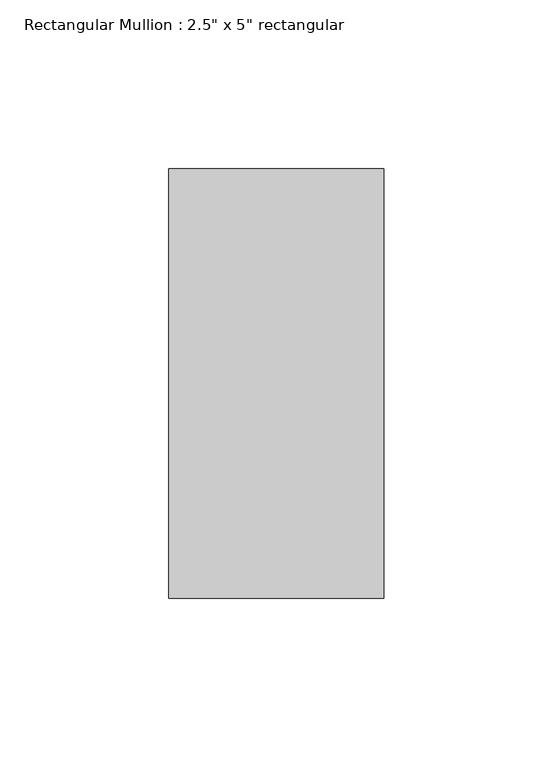
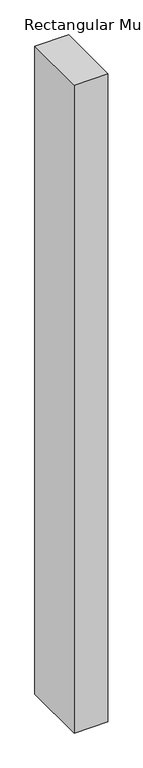
"""IFC4 building model written with IfcOpenShell, lengths in millimetres: member geometry."""

from ifc_helpers import new_model, si_unit, frame, origin, place, context, project, spatial, polyline, outline, extrude, source, transform, mapped, element, save


def member_a1fdef72(model_context):
    return source(origin(), model_context, "Body", "SweptSolid", [
        extrude(outline(polyline([(0.0, 63.5), (0.0, -63.5), (-63.5, -63.5), (-63.5, 63.5), (0.0, 63.5)])), frame((0.0, 0.0, -1282.9185959), z_axis=(0.0, 0.0, 1.0), x_axis=(1.0, 0.0, 0.0)), (0.0, 0.0, 1.0), 1282.9185959),
    ])


if __name__ == "__main__":
    model = new_model("IFC4")
    model_context = context("Model", 3, world=origin())
    ifc_project = project(units=[si_unit("LENGTHUNIT", "METRE", prefix="MILLI")], contexts=[model_context])
    site = spatial("IfcSite", under=ifc_project)
    building = spatial("IfcBuilding", under=site)
    placement = place(None, origin())
    member_shape = member_a1fdef72(model_context)
    element("IfcMember", 1, ObjectType="Rectangular Mullion : 2.5\" x 5\" rectangular", at=placement, inside=building, context=model_context, shape_type="MappedRepresentation", body=[
        mapped(member_shape, transform((0.0, 0.0, 0.0), x_axis=(1.0, 0.0, 0.0), y_axis=(0.0, 1.0, 0.0), z_axis=(0.0, 0.0, 1.0))),
    ])
    save(model, "model.ifc")

# Revit data of these elements
# Type "Rectangular Mullion : 2.5\" x 5\" rectangular"
#   built-in parameter 1007304 = 0.416667 (stored number, unit not read)
#   built-in parameter 1007301 = 0.104167 (stored number, unit not read)
#   built-in parameter 1007300 = 0.104167 (stored number, unit not read)
# Element 1 (IfcMember, "Rectangular Mullion : 2.5\" x 5\" rectangular")
#   Materials on its faces: "Aluminum"
# Materials
#   "Aluminum": class "Metal", colour RGB 247 247 247, transparency 0, Description = "Aluminum 6061", Cost = 0
